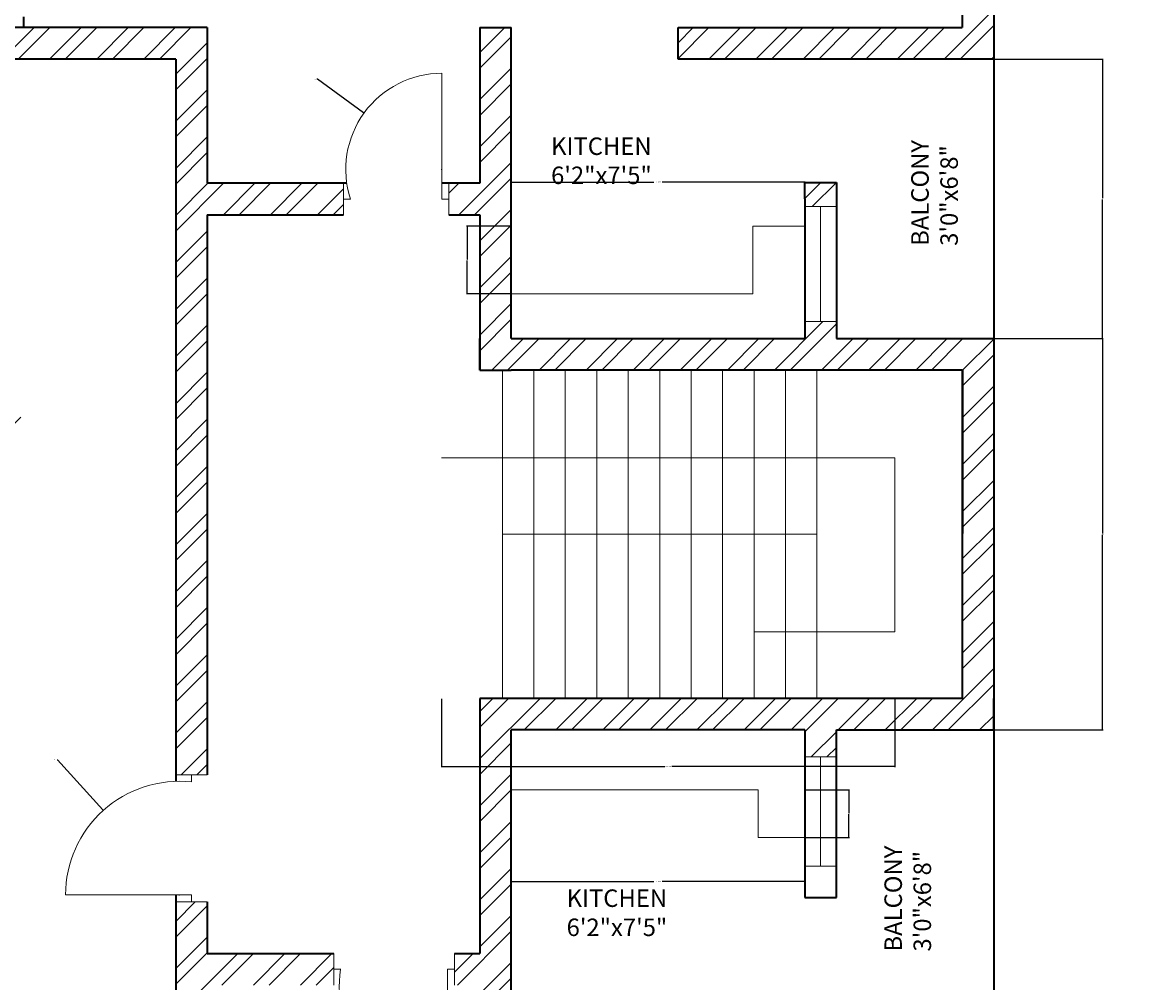
# Model space of a CAD drawing. Units: inches. Extents: x 1955 to 3324, y 980 to 3129.
# Tile 5 of 11: x 2237 to 2555, y 2048 to 2323. Entities that reach past the tile are written whole.
import ezdxf

# ---------------------------------------------------------------- set-up
doc = ezdxf.new("R2010")
doc.units = ezdxf.units.IN
for name, color, linetype, lineweight in [('A-ANNO-DIMS', 2, 'Continuous', 18), ('A-AREA-IDEN', 7, 'Continuous', 18), ('A-DOOR', 3, 'Continuous', 18), ('A-FLOR-CASE', 8, 'Continuous', 18), ('A-FLOR-STRS', 7, 'Continuous', 18), ('A-GLAZ', 4, 'Continuous', 18), ('A-WALL', 7, 'Continuous', 35), ('A-WALL-PATT', 252, 'Continuous', 13)]:
    doc.layers.add(name, color=color, linetype=linetype, lineweight=lineweight)
doc.styles.get("Standard").update_dxf_attribs({"font": 'arial.ttf'})
doc.dimstyles.get("Standard").update_dxf_attribs({"dimtxt": 0.18, "dimasz": 0.18, "dimexe": 0.18, "dimexo": 0.0625, "dimgap": 0.09, "dimtad": 0, "dimtih": 1, "dimtoh": 1, "dimdec": 4, "dimzin": 0, "dimdsep": 46, "dimtxsty": 'Standard', "dimcen": 0.09, "dimadec": 0, "dimazin": 0, "dimtfac": 1, "dimtdec": 4, "dimtofl": 0, "dimtmove": 0, "dimatfit": 3, "dimfxl": 1, "dimtolj": 1, "dimtzin": 0, "dimarcsym": 0})

# ---------------------------------------------------------------- blocks, each defined once
blk = doc.blocks.new('DOOR-UNIT-W')
for p, q in [((31.5, 36.35), (40.5, 36.35)), ((40.5, 36.35), (36, 36.35)), ((36, 36.35), (36, 34.35)), ((36, 2), (0, 2)), ((31.5, 0), (40.5, 0)), ((36, 0), (36, 2)), ((40.5, 0), (36, 0))]:
    blk.add_line(p, q)
blk.add_arc((32.53, 2), 32.53, 83.8799, 180)
blk = doc.blocks.new('DOOR-UNIT-N')
for p, q in [((28.16, 4.5), (28.16, 40.5)), ((0, 9), (0, 0)), ((30.16, 0), (30.16, 9)), ((30.16, 9), (30.16, 4.5)), ((0, 0), (0, 4.5)), ((0, 4.5), (2, 4.5)), ((30.16, 4.5), (28.16, 4.5))]:
    blk.add_line(p, q)
blk.add_arc((28.16, 12.99), 27.51, 90, 197.982)
blk = doc.blocks.new('DOOR-UNIT-S')
for p, q in [((0, 31.5), (0, 40.5)), ((0, 40.5), (0, 36)), ((34.6, 31.5), (34.6, 40.5)), ((34.6, 40.5), (34.6, 36)), ((0, 36), (2, 36)), ((34.6, 36), (32.6, 36)), ((32.6, 36), (32.6, 0))]:
    blk.add_line(p, q)
blk.add_arc((32.6, 31.01), 31.01, 170.7301, 270)
blk = doc.blocks.new('WIN-PLAN-33')
for p, q in [((4.5, 32.88), (0, 32.88)), ((0, 32.88), (9, 32.88)), ((4.5, 0), (4.5, 32.88)), ((0, 0), (9, 0)), ((9, 0), (4.5, 0))]:
    blk.add_line(p, q)
blk = doc.blocks.new('WIN-PLAN-31')
for p, q in [((0, 31.31), (9, 31.31)), ((9, 31.31), (4.5, 31.31)), ((4.5, 31.31), (4.5, 0)), ((4.5, 0), (0, 0)), ((0, 0), (9, 0))]:
    blk.add_line(p, q)
blk = doc.blocks.new('COUNTER-L-N')
for p, q in [((83.99, 19.45), (69.13, 19.45)), ((69.13, 19.45), (69.13, 0)), ((69.13, 0), (0, 0))]:
    blk.add_line(p, q)
blk = doc.blocks.new('COUNTER-L-S')
for p, q in [((0, 13.55), (70.65, 13.55)), ((70.65, 13.55), (70.65, 0)), ((70.65, 0), (83.99, 0))]:
    blk.add_line(p, q)
blk = doc.blocks.new('STAIR-RETURN-FLIGHT')
for p, q in [((17.37, 47), (17.37, 94)), ((17.37, 94), (17.37, 0)), ((26.37, 94), (26.37, 0)), ((35.37, 94), (35.37, 0)), ((44.37, 94), (44.37, 0)), ((53.37, 94), (53.37, 0)), ((62.37, 94), (62.37, 0)), ((71.37, 94), (71.37, 0)), ((80.37, 94), (80.37, 0)), ((89.37, 94), (89.37, 0)), ((98.37, 94), (98.37, 0)), ((107.37, 94), (107.37, 0)), ((0, 68.91), (129.63, 68.91)), ((129.63, 68.91), (129.63, 19.03)), ((107.37, 47), (17.37, 47)), ((129.63, 19.03), (89.37, 19.03))]:
    blk.add_line(p, q)
blk = doc.blocks.new('*D77')
at = {"layer": 'A-ANNO-DIMS', "color": 0, "lineweight": -2, "transparency": 16777216}
for p, q in [((2377.22, 2264.77), (2377.22, 2277.48)), ((2377.4, 2277.3), (2418.03, 2277.3)), ((2461.03, 2277.3), (2420.4, 2277.3)), ((2461.21, 2264.77), (2461.21, 2277.48))]:
    blk.add_line(p, q, dxfattribs=at)
at = {"layer": 'A-ANNO-DIMS', "color": 0, "transparency": 16777216}
for points in [[(2377.4, 2277.33), (2377.4, 2277.27), (2377.22, 2277.3)], [(2461.03, 2277.33), (2461.03, 2277.27), (2461.21, 2277.3)]]:
    blk.add_solid(points, dxfattribs=at)
at = {"layer": 'Defpoints', "color": 0, "transparency": 16777216}
for p in [(2461.21, 2277.3), (2377.22, 2264.71), (2461.21, 2264.71)]:
    blk.add_point(p, dxfattribs=at)
at = {"layer": 'A-ANNO-DIMS', "color": 0, "transparency": 16777216, "insert": (2419.22, 2277.3), "char_height": 0.18, "attachment_point": 5}
blk.add_mtext('\\A1;COUNTER 84 TYP.', dxfattribs=at)
blk = doc.blocks.new('*D78')
at = {"layer": 'A-ANNO-DIMS', "color": 0, "lineweight": -2, "transparency": 16777216}
for p, q in [((2377.16, 2264.71), (2364.44, 2264.71)), ((2364.62, 2264.53), (2364.62, 2255.16)), ((2364.62, 2245.44), (2364.62, 2254.8)), ((2377.16, 2245.26), (2364.44, 2245.26))]:
    blk.add_line(p, q, dxfattribs=at)
at = {"layer": 'A-ANNO-DIMS', "color": 0, "transparency": 16777216}
for points in [[(2364.59, 2264.53), (2364.65, 2264.53), (2364.62, 2264.71)], [(2364.59, 2245.44), (2364.65, 2245.44), (2364.62, 2245.26)]]:
    blk.add_solid(points, dxfattribs=at)
at = {"layer": 'Defpoints', "color": 0, "transparency": 16777216}
for p in [(2364.62, 2264.71), (2377.22, 2264.71), (2377.22, 2245.26)]:
    blk.add_point(p, dxfattribs=at)
at = {"layer": 'A-ANNO-DIMS', "color": 0, "transparency": 16777216, "insert": (2364.62, 2254.98), "char_height": 0.18, "attachment_point": 5}
blk.add_mtext('\\A1;19 TYP.', dxfattribs=at)
blk = doc.blocks.new('*D79')
at = {"layer": 'A-ANNO-DIMS', "color": 0, "lineweight": -2, "transparency": 16777216}
for p, q in [((2377.22, 2089.7), (2377.22, 2076.99)), ((2461.21, 2089.7), (2461.21, 2076.99)), ((2377.4, 2077.17), (2418.03, 2077.17)), ((2461.03, 2077.17), (2420.4, 2077.17))]:
    blk.add_line(p, q, dxfattribs=at)
at = {"layer": 'A-ANNO-DIMS', "color": 0, "transparency": 16777216}
for points in [[(2377.4, 2077.2), (2377.4, 2077.14), (2377.22, 2077.17)], [(2461.03, 2077.2), (2461.03, 2077.14), (2461.21, 2077.17)]]:
    blk.add_solid(points, dxfattribs=at)
at = {"layer": 'Defpoints', "color": 0, "transparency": 16777216}
for p in [(2377.22, 2089.76), (2461.21, 2089.76), (2461.21, 2077.17)]:
    blk.add_point(p, dxfattribs=at)
at = {"layer": 'A-ANNO-DIMS', "color": 0, "transparency": 16777216, "insert": (2419.22, 2077.17), "char_height": 0.18, "attachment_point": 5}
blk.add_mtext('\\A1;COUNTER 84 TYP.', dxfattribs=at)
blk = doc.blocks.new('*D80')
at = {"layer": 'A-ANNO-DIMS', "color": 0, "lineweight": -2, "transparency": 16777216}
for p, q in [((2461.27, 2103.32), (2473.99, 2103.32)), ((2473.81, 2103.14), (2473.81, 2096.72)), ((2473.81, 2089.94), (2473.81, 2096.36)), ((2461.27, 2089.76), (2473.99, 2089.76))]:
    blk.add_line(p, q, dxfattribs=at)
at = {"layer": 'A-ANNO-DIMS', "color": 0, "transparency": 16777216}
for points in [[(2473.78, 2103.14), (2473.84, 2103.14), (2473.81, 2103.32)], [(2473.78, 2089.94), (2473.84, 2089.94), (2473.81, 2089.76)]]:
    blk.add_solid(points, dxfattribs=at)
at = {"layer": 'Defpoints', "color": 0, "transparency": 16777216}
for p in [(2461.21, 2103.32), (2473.81, 2103.32), (2461.21, 2089.76)]:
    blk.add_point(p, dxfattribs=at)
at = {"layer": 'A-ANNO-DIMS', "color": 0, "transparency": 16777216, "insert": (2473.81, 2096.54), "char_height": 0.18, "attachment_point": 5}
blk.add_mtext('\\A1;14 TYP.', dxfattribs=at)
blk = doc.blocks.new('*D83')
at = {"layer": 'A-ANNO-DIMS', "color": 0, "lineweight": -2, "transparency": 16777216}
for p, q in [((2357.29, 2129.44), (2357.29, 2109.88)), ((2486.92, 2129.44), (2486.92, 2109.88)), ((2357.47, 2110.06), (2421.11, 2110.06)), ((2486.74, 2110.06), (2423.11, 2110.06))]:
    blk.add_line(p, q, dxfattribs=at)
at = {"layer": 'A-ANNO-DIMS', "color": 0, "transparency": 16777216}
for points in [[(2357.47, 2110.09), (2357.47, 2110.03), (2357.29, 2110.06)], [(2486.74, 2110.09), (2486.74, 2110.03), (2486.92, 2110.06)]]:
    blk.add_solid(points, dxfattribs=at)
at = {"layer": 'Defpoints', "color": 0, "transparency": 16777216}
for p in [(2357.29, 2129.5), (2486.92, 2129.5), (2486.92, 2110.06)]:
    blk.add_point(p, dxfattribs=at)
at = {"layer": 'A-ANNO-DIMS', "color": 0, "transparency": 16777216, "insert": (2422.11, 2110.06), "char_height": 0.18, "attachment_point": 5}
blk.add_mtext('\\A1;STAIR 130 TYP.', dxfattribs=at)
blk = doc.blocks.new('*D84')
at = {"layer": 'A-ANNO-DIMS', "color": 0, "lineweight": -2, "transparency": 16777216}
for p, q in [((2486.98, 2223.5), (2506.55, 2223.5)), ((2506.37, 2223.32), (2506.37, 2176.69)), ((2506.37, 2129.68), (2506.37, 2176.32)), ((2486.98, 2129.5), (2506.55, 2129.5))]:
    blk.add_line(p, q, dxfattribs=at)
at = {"layer": 'A-ANNO-DIMS', "color": 0, "transparency": 16777216}
for points in [[(2506.34, 2223.32), (2506.4, 2223.32), (2506.37, 2223.5)], [(2506.34, 2129.68), (2506.4, 2129.68), (2506.37, 2129.5)]]:
    blk.add_solid(points, dxfattribs=at)
at = {"layer": 'Defpoints', "color": 0, "transparency": 16777216}
for p in [(2486.92, 2223.5), (2506.37, 2223.5), (2486.92, 2129.5)]:
    blk.add_point(p, dxfattribs=at)
at = {"layer": 'A-ANNO-DIMS', "color": 0, "transparency": 16777216, "insert": (2506.37, 2176.5), "char_height": 0.18, "attachment_point": 5}
blk.add_mtext('\\A1;94 TYP.', dxfattribs=at)
blk = doc.blocks.new('*D103')
at = {"layer": 'A-ANNO-DIMS', "color": 0, "lineweight": -2, "transparency": 16777216}
for p, q in [((2515.27, 2312.5), (2546.54, 2312.5)), ((2546.36, 2312.32), (2546.36, 2272.69)), ((2546.36, 2232.68), (2546.36, 2272.32)), ((2515.27, 2232.5), (2546.54, 2232.5))]:
    blk.add_line(p, q, dxfattribs=at)
at = {"layer": 'A-ANNO-DIMS', "color": 0, "transparency": 16777216}
for points in [[(2546.33, 2312.32), (2546.39, 2312.32), (2546.36, 2312.5)], [(2546.33, 2232.68), (2546.39, 2232.68), (2546.36, 2232.5)]]:
    blk.add_solid(points, dxfattribs=at)
at = {"layer": 'Defpoints', "color": 0, "transparency": 16777216}
for p in [(2515.21, 2312.5), (2546.36, 2312.5), (2515.21, 2232.5)]:
    blk.add_point(p, dxfattribs=at)
at = {"layer": 'A-ANNO-DIMS', "color": 0, "transparency": 16777216, "insert": (2546.36, 2272.5), "char_height": 0.18, "attachment_point": 5}
blk.add_mtext('\\A1;80', dxfattribs=at)
blk = doc.blocks.new('*D104')
at = {"layer": 'A-ANNO-DIMS', "color": 0, "lineweight": -2, "transparency": 16777216}
for p, q in [((2515.27, 2232.5), (2546.54, 2232.5)), ((2546.36, 2232.32), (2546.36, 2176.68)), ((2546.36, 2120.68), (2546.36, 2176.32)), ((2515.27, 2120.5), (2546.54, 2120.5))]:
    blk.add_line(p, q, dxfattribs=at)
at = {"layer": 'A-ANNO-DIMS', "color": 0, "transparency": 16777216}
for points in [[(2546.33, 2232.32), (2546.39, 2232.32), (2546.36, 2232.5)], [(2546.33, 2120.68), (2546.39, 2120.68), (2546.36, 2120.5)]]:
    blk.add_solid(points, dxfattribs=at)
at = {"layer": 'Defpoints', "color": 0, "transparency": 16777216}
for p in [(2515.21, 2232.5), (2546.36, 2232.5), (2515.21, 2120.5)]:
    blk.add_point(p, dxfattribs=at)
at = {"layer": 'A-ANNO-DIMS', "color": 0, "transparency": 16777216, "insert": (2546.36, 2176.5), "char_height": 0.18, "attachment_point": 5}
blk.add_mtext('\\A1;112', dxfattribs=at)
blk = doc.blocks.new('*D139')
at = {"layer": 'A-ANNO-DIMS', "color": 0, "lineweight": -2, "transparency": 16777216}
for p, q in [((2247.27, 2111.99), (2247.45, 2111.99)), ((2247.45, 2111.99), (2260.38, 2097.6)), ((2282.15, 2073.27), (2282.33, 2073.27)), ((2282.24, 2073.18), (2282.24, 2073.36))]:
    blk.add_line(p, q, dxfattribs=at)
at = {"layer": 'A-ANNO-DIMS', "color": 0, "transparency": 16777216}
blk.add_solid([(2260.4, 2097.62), (2260.36, 2097.58), (2260.5, 2097.47)], dxfattribs=at)
at = {"layer": 'Defpoints', "color": 0, "transparency": 16777216}
for p in [(2260.5, 2097.47), (2282.24, 2073.27)]:
    blk.add_point(p, dxfattribs=at)
at = {"layer": 'A-ANNO-DIMS', "color": 0, "transparency": 16777216, "insert": (2246.79, 2111.99), "char_height": 0.18, "attachment_point": 5}
blk.add_mtext('\\A1;R32.53', dxfattribs=at)
blk = doc.blocks.new('*D143')
at = {"layer": 'A-ANNO-DIMS', "color": 0, "lineweight": -2, "transparency": 16777216}
for p, q in [((2321.6, 2306.8), (2321.78, 2306.8)), ((2321.78, 2306.8), (2334.98, 2297.2)), ((2357.29, 2280.92), (2357.47, 2280.92)), ((2357.38, 2280.83), (2357.38, 2281.01))]:
    blk.add_line(p, q, dxfattribs=at)
at = {"layer": 'A-ANNO-DIMS', "color": 0, "transparency": 16777216}
blk.add_solid([(2335, 2297.22), (2334.96, 2297.17), (2335.13, 2297.09)], dxfattribs=at)
at = {"layer": 'Defpoints', "color": 0, "transparency": 16777216}
for p in [(2335.13, 2297.09), (2357.38, 2280.92)]:
    blk.add_point(p, dxfattribs=at)
at = {"layer": 'A-ANNO-DIMS', "color": 0, "transparency": 16777216, "insert": (2321.13, 2306.8), "char_height": 0.18, "attachment_point": 5}
blk.add_mtext('\\A1;R27.51', dxfattribs=at)

msp = doc.modelspace()

# ---------------------------------------------------------------- hatches: boundary and pattern name
at = {"layer": 'A-WALL-PATT'}
h = msp.add_hatch(dxfattribs=at)
h.set_pattern_fill('ANSI32', color=256)
h.paths.add_polyline_path([(2361.4775, 2456.5037), (2270.2755, 2456.5037), (2270.2755, 2447.5037), (2285.7102, 2447.5037), (2285.7102, 2363.5037), (2281.1795, 2363.5037), (2281.1795, 2359.0037), (2290.2102, 2359.0037), (2290.2102, 2447.5037), (2361.4775, 2447.5037), (2361.4775, 2452.0037)])
h.paths.add_polyline_path([(2246.2755, 2456.5037), (2197.6809, 2456.5037), (2197.6809, 2447.5037), (2233.2102, 2447.5037), (2233.2102, 2355.6044), (2237.7102, 2355.6044), (2237.7102, 2447.5037), (2246.2755, 2447.5037)], flags=17)
h.paths.add_polyline_path([(2137.6809, 2456.5037), (2110.2102, 2456.5037), (2110.2102, 2312.5037), (2152.2102, 2312.5037), (2281.2102, 2312.5037), (2281.2102, 2107.6185), (2290.2102, 2107.6185), (2290.2102, 2267.9289), (2329.216, 2267.9289), (2329.216, 2272.4289), (2329.216, 2276.9289), (2290.2102, 2276.9289), (2290.2102, 2321.5037), (2281.2102, 2321.5037), (2119.2102, 2321.5037), (2119.2102, 2447.5037), (2137.6809, 2447.5037)])
h.paths.add_polyline_path([(2515.2102, 2456.5037), (2421.4775, 2456.5037), (2421.4775, 2447.5037), (2506.2102, 2447.5037), (2506.2102, 2415.6626), (2515.2102, 2415.6626)])
h.paths.add_polyline_path([(2515.2102, 2355.6626), (2506.2102, 2355.6626), (2506.2102, 2321.5037), (2424.9282, 2321.5037), (2424.9282, 2312.5037), (2461.2102, 2312.5037), (2470.2102, 2312.5037), (2515.2102, 2312.5037)])
h.paths.add_polyline_path([(2515.2102, 2232.5037), (2470.2102, 2232.5037), (2470.2102, 2237.3759), (2465.7102, 2237.3759), (2461.2102, 2237.3759), (2461.2102, 2232.5037), (2377.2219, 2232.5037), (2377.2219, 2321.5037), (2368.2219, 2321.5037), (2368.2219, 2276.9289), (2359.3802, 2276.9289), (2359.3802, 2272.4289), (2359.3802, 2267.9289), (2368.2219, 2267.9289), (2368.2219, 2223.5037), (2377.2219, 2223.5037), (2461.2102, 2223.5037), (2506.2102, 2223.5037), (2506.2102, 2129.5037), (2461.2102, 2129.5037), (2387.2102, 2129.5037), (2368.2219, 2129.5037), (2368.2219, 2056.4936), (2361.0095, 2056.4936), (2361.0095, 2051.9936), (2361.0095, 2047.4936), (2368.2219, 2047.4936), (2368.2219, 2031.5037), (2377.2219, 2031.5037), (2377.2219, 2120.5037), (2461.2102, 2120.5037), (2461.2102, 2112.7921), (2470.2102, 2112.7921), (2470.2102, 2120.5037), (2515.2102, 2120.5037), (2515.2102, 2129.5037)])
h.paths.add_polyline_path([(2470.2102, 2277.1758), (2461.2102, 2277.1758), (2461.2102, 2272.5037), (2461.2102, 2270.2549), (2470.2102, 2270.2549), (2470.2102, 2272.5037)], flags=17)
h.paths.add_polyline_path([(2515.2102, 2040.5037), (2470.2102, 2040.5037), (2417.8264, 2040.5037), (2417.8264, 2031.5037), (2506.2102, 2031.5037), (2506.2102, 2005.3639), (2515.2102, 2005.3639)])
h.paths.add_polyline_path([(2506.2102, 1905.5037), (2402.6963, 1905.5037), (2402.6963, 1896.5037), (2506.2102, 1896.5037)])
h.paths.add_polyline_path([(2515.2102, 1945.3639), (2506.2102, 1945.3639), (2506.2102, 1905.5037), (2506.2102, 1896.5037), (2515.2102, 1896.5037)])
h.paths.add_polyline_path([(2342.6963, 1901.0037), (2342.6963, 1905.5037), (2273.4892, 1905.5037), (2273.4892, 1896.5037), (2342.6963, 1896.5037)])
h.paths.add_polyline_path([(2290.2102, 1994.0037), (2283.612, 1994.0037), (2283.612, 1991.7537), (2283.612, 1989.5037), (2285.7102, 1989.5037), (2285.7102, 1905.5037), (2290.2102, 1905.5037)])
h.paths.add_polyline_path([(2249.4892, 1905.5037), (2237.7102, 1905.5037), (2206.3617, 1905.5037), (2206.3617, 1896.5037), (2249.4892, 1896.5037), (2249.4892, 1901.0037)])
h.paths.add_polyline_path([(2237.7102, 1989.5037), (2261.7102, 1989.5037), (2261.7102, 1994.0037), (2237.7102, 1994.0037), (2237.7102, 1999.266), (2235.4602, 1999.266), (2233.2102, 1999.266), (2233.2102, 1994.0037), (2233.2102, 1905.5037), (2237.7102, 1905.5037)])
h.paths.add_polyline_path([(2119.2102, 1947.5144), (2110.2102, 1947.5144), (2110.2102, 1896.5037), (2119.2102, 1896.5037), (2146.3617, 1896.5037), (2146.3617, 1901.0037), (2146.3617, 1905.5037), (2119.2102, 1905.5037)])
h.paths.add_polyline_path([(2119.2102, 2068.6379), (2110.2102, 2068.6379), (2110.2102, 2007.5144), (2119.2102, 2007.5144), (2119.2102, 2031.5037), (2233.2102, 2031.5037), (2233.2102, 2027.9287), (2235.4602, 2027.9287), (2237.7102, 2027.9287), (2237.7102, 2031.5037), (2281.2102, 2031.5037), (2290.2102, 2031.5037), (2290.2102, 2047.4936), (2326.409, 2047.4936), (2326.409, 2056.4936), (2290.2102, 2056.4936), (2290.2102, 2071.2722), (2285.7102, 2071.2722), (2281.2102, 2071.2722), (2281.2102, 2040.5037), (2227.2102, 2040.5037), (2227.2102, 2111.2571), (2222.7102, 2111.2571), (2218.2102, 2111.2571), (2218.2102, 2040.5037), (2119.2102, 2040.5037)])
h.paths.add_polyline_path([(2236.9166, 2214.5037), (2161.2102, 2214.5037), (2161.2102, 2221.6488), (2152.2102, 2221.6488), (2152.2102, 2214.5037), (2110.2102, 2214.5037), (2110.2102, 2205.5037), (2131.2394, 2205.5037), (2131.2394, 2198.3478), (2140.2394, 2198.3478), (2140.2394, 2205.5037), (2224.2394, 2205.5037), (2224.2394, 2200.2317), (2228.7394, 2200.2317), (2233.2394, 2200.2317), (2233.2394, 2205.5037), (2236.9166, 2205.5037)], flags=17)
h.paths.add_polyline_path([(2236.9166, 2157.5037), (2233.2394, 2157.5037), (2233.2394, 2178.9172), (2228.7394, 2178.9172), (2224.2394, 2178.9172), (2224.2394, 2157.5037), (2140.2394, 2157.5037), (2140.2394, 2174.3478), (2131.2394, 2174.3478), (2131.2394, 2157.5037), (2110.2102, 2157.5037), (2110.2102, 2128.6379), (2119.2102, 2128.6379), (2119.2102, 2148.5037), (2218.2102, 2148.5037), (2218.2102, 2141.7262), (2222.7102, 2141.7262), (2227.2102, 2141.7262), (2227.2102, 2148.5037), (2236.9166, 2148.5037)], flags=0)
h.paths.add_polyline_path([(3084.7449, 2537.3808), (3212.7954, 2537.3808), (3212.7954, 2555.9271), (3084.7449, 2555.9271)], flags=9)
h.paths.add_polyline_path([(3068.7485, 2853.43), (3169.977, 2853.43), (3169.977, 2871.9764), (3068.7485, 2871.9764)], flags=9)
h.paths.add_polyline_path([(3074.1798, 2918.0252), (3126.4732, 2918.0252), (3126.4732, 2936.5716), (3074.1798, 2936.5716)], flags=9)
h.paths.add_polyline_path([(3073.0928, 2947.3127), (3199.0499, 2947.3127), (3199.0499, 2965.8591), (3073.0928, 2965.8591)], flags=9)
h.paths.add_polyline_path([(2733.8393, 2484.8678), (2879.7915, 2484.8678), (2879.7915, 2521.9606), (2733.8393, 2521.9606)], flags=9)
h.paths.add_polyline_path([(2204.9881, 2482.4168), (2355.1272, 2482.4168), (2355.1272, 2519.5095), (2204.9881, 2519.5095)], flags=9)
h.paths.add_polyline_path([(3062.1429, 2387.2466), (3079.3735, 2387.2466), (3079.3735, 2411.9751), (3062.1429, 2411.9751)], flags=9)
h.paths.add_polyline_path([(2190.1574, 2158.8439), (2219.315, 2158.8439), (2219.315, 2177.5013), (2190.1574, 2177.5013)], flags=25)
h.paths.add_polyline_path([(2213.6766, 1840.7276), (2405.0382, 1840.7276), (2405.0382, 1865.4561), (2213.6766, 1865.4561)], flags=9)
h.paths.add_polyline_path([(2180.5398, 2233.911), (2213.9471, 2233.911), (2213.9471, 2252.5683), (2180.5398, 2252.5683)], flags=25)
h.paths.add_polyline_path([(2134.4484, 2238.3973), (2134.4484, 2274.2807), (2115.791, 2274.2807), (2115.791, 2238.3973)], flags=25)
h.paths.add_polyline_path([(2135.1593, 2122.9991), (2173.7507, 2122.9991), (2173.7507, 2141.6565), (2135.1593, 2141.6565)], flags=25)
h.paths.add_polyline_path([(2129.8822, 2002.1912), (2168.4736, 2002.1912), (2168.4736, 2020.8486), (2129.8822, 2020.8486)], flags=9)
h.paths.add_polyline_path([(2239.6647, 1953.4107), (2268.8973, 1953.4107), (2268.8973, 1972.068), (2239.6647, 1972.068)], flags=9)
h.paths.add_polyline_path([(2352.8562, 1951.2904), (2402.1775, 1951.2904), (2402.1775, 1969.9477), (2352.8562, 1969.9477)], flags=9)
h.paths.add_polyline_path([(2500.1358, 2055.32), (2500.1358, 2091.2034), (2481.4784, 2091.2034), (2481.4784, 2055.32)], flags=25)
h.paths.add_polyline_path([(2391.2702, 2058.6821), (2424.4285, 2058.6821), (2424.4285, 2077.3394), (2391.2702, 2077.3394)], flags=25)
h.paths.add_polyline_path([(2507.7996, 2257.2758), (2507.7996, 2293.1592), (2489.1422, 2293.1592), (2489.1422, 2257.2758)], flags=25)
h.paths.add_polyline_path([(2386.8349, 2273.8734), (2419.9931, 2273.8734), (2419.9931, 2292.5307), (2386.8349, 2292.5307)], flags=25)
h.paths.add_polyline_path([(2335.374, 2373.3267), (2384.6953, 2373.3267), (2384.6953, 2391.984), (2335.374, 2391.984)], flags=9)
h.paths.add_polyline_path([(2243.8205, 2380.6539), (2273.0531, 2380.6539), (2273.0531, 2399.3113), (2243.8205, 2399.3113)], flags=25)
h.paths.add_polyline_path([(2126.2627, 2321.6894), (2164.8541, 2321.6894), (2164.8541, 2340.3467), (2126.2627, 2340.3467)], flags=25)

# ---------------------------------------------------------------- linework, layer by layer
at = {"layer": 'A-WALL'}
for p, q in [((2515.2102, 2456.5037), (2515.2102, 1896.5037)), ((2506.2102, 2447.5037), (2506.2102, 2321.5037)), ((2237.7102, 2324.5535), (2237.7102, 2321.5037)), ((2290.2102, 2321.5037), (2119.2102, 2321.5037)), ((2290.2102, 2321.5037), (2281.2102, 2321.5037)), ((2290.2102, 2321.5037), (2290.2102, 2276.9289)), ((2368.2219, 2321.5037), (2377.2219, 2321.5037)), ((2368.2219, 2321.5037), (2368.2219, 2276.9289)), ((2377.2219, 2232.5037), (2377.2219, 2321.5037)), ((2424.9282, 2312.5037), (2424.9282, 2321.5037)), ((2424.9282, 2321.5037), (2506.2102, 2321.5037)), ((2281.2102, 2312.5037), (2110.2102, 2312.5037)), ((2281.2102, 2312.5037), (2281.2102, 2105.7875)), ((2461.2102, 2312.5037), (2424.9282, 2312.5037)), ((2470.2102, 2312.5037), (2461.2102, 2312.5037)), ((2515.2102, 2312.5037), (2470.2102, 2312.5037)), ((2330.1636, 2276.9289), (2290.2102, 2276.9289)), ((2368.2219, 2276.9289), (2357.3802, 2276.9289)), ((2461.2102, 2272.5037), (2461.2102, 2277.1758)), ((2461.2102, 2277.1758), (2470.2102, 2277.1758)), ((2470.2102, 2277.1758), (2470.2102, 2272.5037)), ((2461.2102, 2272.5037), (2461.2102, 2232.5037)), ((2470.2102, 2272.5037), (2470.2102, 2232.5037)), ((2290.2102, 2267.9289), (2329.216, 2267.9289)), ((2290.2102, 2267.9289), (2290.2102, 2107.6185)), ((2359.3802, 2267.9289), (2368.2219, 2267.9289)), ((2368.2219, 2267.9289), (2368.2219, 2223.5037)), ((2368.2219, 2223.5037), (2368.2219, 2232.5037)), ((2377.2219, 2232.5037), (2461.2102, 2232.5037)), ((2470.2102, 2232.5037), (2515.2102, 2232.5037)), ((2368.2219, 2228.0037), (2368.2219, 2223.5037)), ((2368.2219, 2223.5037), (2377.2219, 2223.5037)), ((2461.2102, 2223.5037), (2377.2219, 2223.5037)), ((2506.2102, 2223.5037), (2461.2102, 2223.5037)), ((2506.2102, 2223.5037), (2506.2102, 2129.5037)), ((2387.2102, 2129.5037), (2368.2219, 2129.5037)), ((2368.2219, 2129.5037), (2368.2219, 2056.4936)), ((2461.2102, 2129.5037), (2387.2102, 2129.5037)), ((2506.2102, 2129.5037), (2461.2102, 2129.5037)), ((2515.2102, 2120.5037), (2515.2102, 2129.5037)), ((2377.2219, 2031.5037), (2377.2219, 2120.5037)), ((2461.2102, 2120.5037), (2377.2219, 2120.5037)), ((2461.2102, 2120.5037), (2461.2102, 2082.2622)), ((2470.2102, 2082.2622), (2470.2102, 2120.5037)), ((2470.2102, 2120.5037), (2515.2102, 2120.5037)), ((2461.2102, 2082.2622), (2461.2102, 2072.5144)), ((2470.2102, 2072.5144), (2470.2102, 2082.2622)), ((2281.2102, 2073.2722), (2281.2102, 2040.5037)), ((2290.2102, 2071.2722), (2290.2102, 2056.4936)), ((2461.2102, 2072.5144), (2470.2102, 2072.5144)), ((2290.2102, 2056.4936), (2326.409, 2056.4936)), ((2361.0095, 2056.4936), (2368.2219, 2056.4936))]:
    msp.add_line(p, q, dxfattribs=at)

# ---------------------------------------------------------------- block references
at = {"layer": 'A-DOOR'}
for name, p in [('DOOR-UNIT-N', (2329.216, 2267.929)), ('DOOR-UNIT-W', (2249.71, 2071.272)), ('DOOR-UNIT-S', (2326.409, 2015.994))]:
    msp.add_blockref(name, p, dxfattribs=at)
at = {"layer": 'A-FLOR-CASE'}
for name, p in [('COUNTER-L-N', (2377.222, 2245.258)), ('COUNTER-L-S', (2377.222, 2089.764))]:
    msp.add_blockref(name, p, dxfattribs=at)
at = {"layer": 'A-FLOR-STRS'}
msp.add_blockref('STAIR-RETURN-FLIGHT', (2357.294, 2129.504), dxfattribs=at)
at = {"layer": 'A-GLAZ'}
for name, p in [('WIN-PLAN-33', (2461.21, 2237.376)), ('WIN-PLAN-31', (2461.21, 2081.487))]:
    msp.add_blockref(name, p, dxfattribs=at)

# ---------------------------------------------------------------- texts
at = {"layer": 'A-AREA-IDEN', "char_height": 5, "attachment_point": 1}
for width, insert in [(107.742202, (2388.5965, 2290.0427)), (92.553247, (2393.0318, 2074.8514))]:
    msp.add_mtext_dynamic_manual_height_columns('KITCHEN\\P6\'2"x7\'5"', width=width, gutter_width=12.5, heights=[0], dxfattribs=dict(at, insert=insert))
at = {"layer": 'A-AREA-IDEN', "char_height": 5, "attachment_point": 1, "rotation": 90}
for width, insert in [(135.361827, (2491.6269, 2259.0374)), (87.248838, (2483.9631, 2057.0816))]:
    msp.add_mtext_dynamic_manual_height_columns('BALCONY\\P3\'0"x6\'8"', width=width, gutter_width=12.5, heights=[0], dxfattribs=dict(at, insert=insert))

# ---------------------------------------------------------------- dimensions: what is measured, and where the dimension line sits
at = {"layer": 'A-ANNO-DIMS'}
for base, p1, p2, picture, middle in [((2546.3602, 2312.5037), (2515.2102, 2232.5037), (2515.2102, 2312.5037), '*D103', (2546.3602, 2272.5037)), ((2546.3602, 2232.5037), (2515.2102, 2120.5037), (2515.2102, 2232.5037), '*D104', (2546.3602, 2176.5037))]:
    dim = msp.add_linear_dim(base=base, p1=p1, p2=p2, angle=90, dimstyle='Standard', override={"dimdec": 0, "dimlfac": 1, "dimrnd": 0, "dimzin": 0, "dimdsep": 46, "dimlunit": 2}, dxfattribs=at)
    dim.commit()
    dim.dimension.update_dxf_attribs({"geometry": picture, "text_midpoint": middle})
for center, mpoint, picture, middle in [((2357.3802, 2280.921), (2335.1282, 2297.0929), '*D143', (2321.1345, 2306.796)), ((2282.2419, 2073.2722), (2260.4993, 2097.4707), '*D139', (2246.7938, 2111.9898))]:
    dim = msp.add_radius_dim(center=center, mpoint=mpoint, dimstyle='Standard', override={"dimdec": 2, "dimlfac": 1, "dimrnd": 0, "dimzin": 0, "dimdsep": 46, "dimlunit": 2}, dxfattribs=at)
    dim.commit()
    dim.dimension.update_dxf_attribs({"geometry": picture, "text_midpoint": middle, "dimtype": 164})
for base, p1, p2, text, picture, middle in [((2461.2102, 2277.3046), (2377.2219, 2264.7063), (2461.2102, 2264.7063), 'COUNTER <> TYP.', '*D77', (2419.216, 2277.3046)), ((2486.9216, 2110.0596), (2357.2941, 2129.5037), (2486.9216, 2129.5037), 'STAIR <> TYP.', '*D83', (2422.1078, 2110.0596)), ((2461.2102, 2077.1656), (2377.2219, 2089.7638), (2461.2102, 2089.7638), 'COUNTER <> TYP.', '*D79', (2419.216, 2077.1656))]:
    dim = msp.add_linear_dim(base=base, p1=p1, p2=p2, text=text, dimstyle='Standard', override={"dimdec": 0, "dimlfac": 1, "dimrnd": 0, "dimzin": 0, "dimdsep": 46, "dimlunit": 2}, dxfattribs=at)
    dim.commit()
    dim.dimension.update_dxf_attribs({"geometry": picture, "text_midpoint": middle})
for base, p1, p2, picture, middle in [((2364.6236, 2264.7063), (2377.2219, 2245.2584), (2377.2219, 2264.7063), '*D78', (2364.6236, 2254.9823)), ((2506.3657, 2223.5037), (2486.9216, 2129.5037), (2486.9216, 2223.5037), '*D84', (2506.3657, 2176.5037)), ((2473.8085, 2103.3156), (2461.2102, 2089.7638), (2461.2102, 2103.3156), '*D80', (2473.8085, 2096.5397))]:
    dim = msp.add_linear_dim(base=base, p1=p1, p2=p2, angle=90, text='<> TYP.', dimstyle='Standard', override={"dimdec": 0, "dimlfac": 1, "dimrnd": 0, "dimzin": 0, "dimdsep": 46, "dimlunit": 2}, dxfattribs=at)
    dim.commit()
    dim.dimension.update_dxf_attribs({"geometry": picture, "text_midpoint": middle})

doc.saveas('drawing.dxf')
